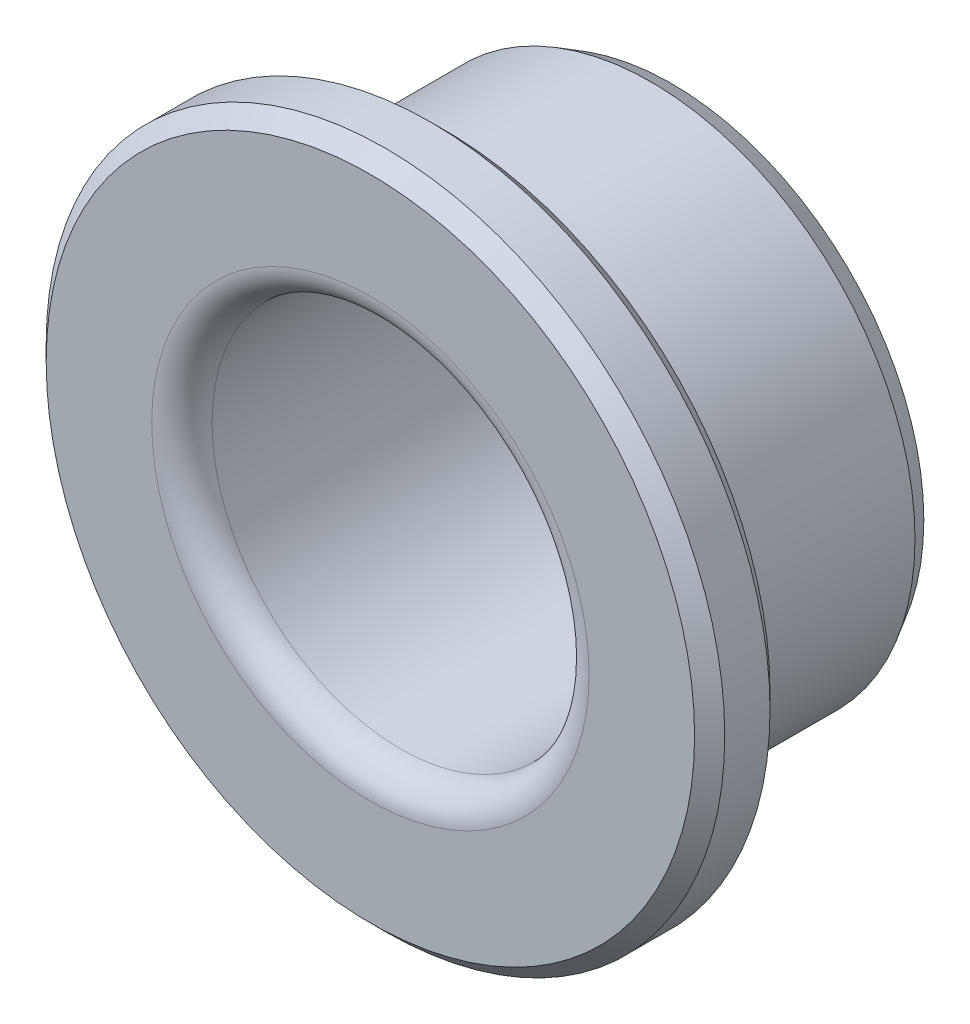
from build123d import *

# Parameters (mm, degrees)
BODY_PROFILE_35_R             = 17.5
BODY_35_DEPTH                 = 15
FLANGE_PROFILE_45_R           = 22.5
FLANGE_45_DEPTH               = 5
BODY_END_CHAMFER_0_8X60_SIZE  = 0.8
BODY_END_CHAMFER_0_8X60_SIZE2 = 1.385640646
BORE_PROFILE_25_R             = 12.5
BORE_25_DEPTH                 = 38.583240946
FLANGE_BORE_FILLET_R2_R       = 2
FLANGE_EDGE_CHAMFER_1X45_SIZE = 1
BODY_BORE_FILLET_R1_R         = 1


with BuildPart() as part:
    # Body Profile Ø35 → Body Ø35 (new body)
    with BuildSketch(Plane.XY):
        Circle(BODY_PROFILE_35_R)
    extrude(amount=BODY_35_DEPTH)

    # Flange Profile Ø45 → Flange Ø45 (add)
    with BuildSketch(Plane.XY.offset(15)):
        Circle(FLANGE_PROFILE_45_R)
    extrude(amount=FLANGE_45_DEPTH)

    # Body End Chamfer 0.8x60°
    body_end_chamfer_0_8x60_edges = [part.edges().sort_by_distance(p)[0] for p in [
        (-17.5, 0, 0),
    ]]
    body_end_chamfer_0_8x60_side = [part.faces().sort_by_distance(p)[0] for p in [
        (0, 0, 0),
    ]]
    chamfer(body_end_chamfer_0_8x60_edges, length=BODY_END_CHAMFER_0_8X60_SIZE, length2=BODY_END_CHAMFER_0_8X60_SIZE2, reference=body_end_chamfer_0_8x60_side[0])

    # Bore Profile Ø25 → Bore Ø25 (cut, through all)
    with BuildSketch(Plane.XY.offset(20)):
        Circle(BORE_PROFILE_25_R)
    extrude(amount=-BORE_25_DEPTH, mode=Mode.SUBTRACT)

    # Flange Bore Fillet R2
    flange_bore_fillet_r2_edges = [part.edges().sort_by_distance(p)[0] for p in [
        (-12.5, 0, 20),
    ]]
    fillet(flange_bore_fillet_r2_edges, radius=FLANGE_BORE_FILLET_R2_R)

    # Flange Edge Chamfer 1x45°
    flange_edge_chamfer_1x45_edges = [part.edges().sort_by_distance(p)[0] for p in [
        (-22.5, 0, 15),
        (-22.5, 0, 20),
    ]]
    chamfer(flange_edge_chamfer_1x45_edges, length=FLANGE_EDGE_CHAMFER_1X45_SIZE)

    # Body Bore Fillet R1
    body_bore_fillet_r1_edges = [part.edges().sort_by_distance(p)[0] for p in [
        (-12.5, 0, 0),
    ]]
    fillet(body_bore_fillet_r1_edges, radius=BODY_BORE_FILLET_R1_R)


solid = part.part
